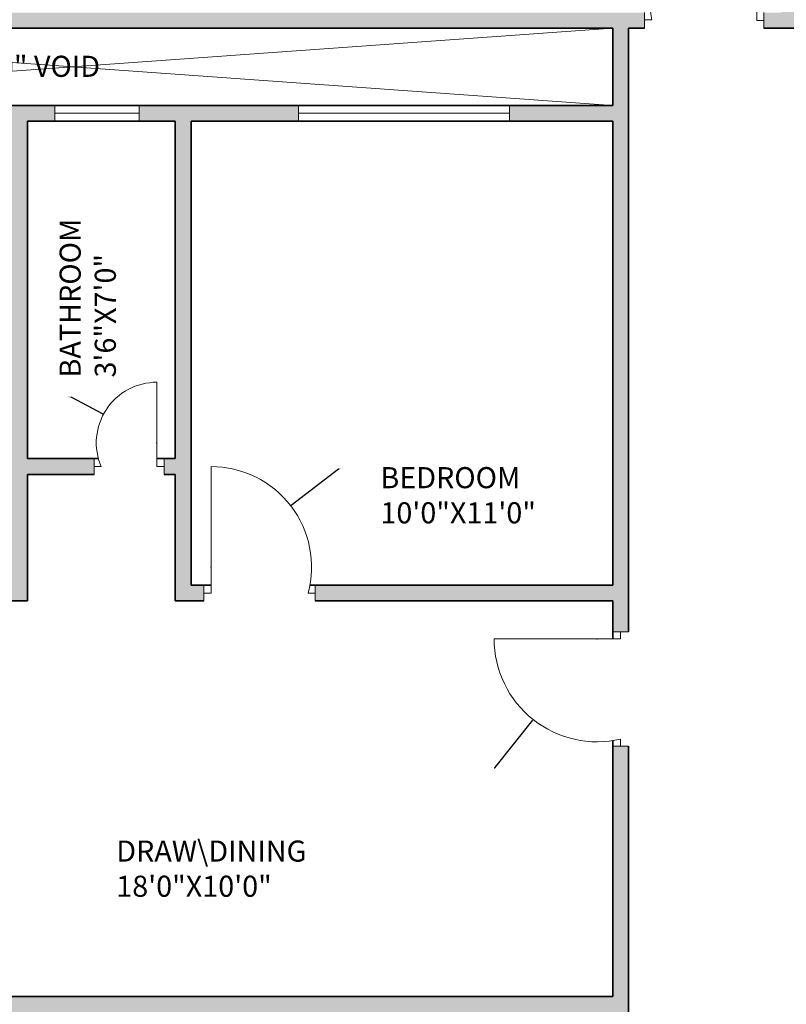
# Model space of a CAD drawing. Units: inches. Extents: x 2314 to 3223, y 1382 to 2735.
# Tile 7 of 14: x 2549 to 2767, y 1864 to 2144. Entities that reach past the tile are written whole.
import ezdxf

# ---------------------------------------------------------------- set-up
doc = ezdxf.new("R2010")
doc.units = ezdxf.units.IN
for name, color, linetype, lineweight in [('A-ANNO-DIMS', 2, 'Continuous', 18), ('A-AREA-IDEN', 7, 'Continuous', 18), ('A-DOOR', 3, 'Continuous', 18), ('A-FLOR-OPEN', 8, 'Continuous', 13), ('A-GLAZ', 4, 'Continuous', 18), ('A-WALL', 7, 'Continuous', 35)]:
    doc.layers.add(name, color=color, linetype=linetype, lineweight=lineweight)
doc.layers.add('A-WALL-PATT', color=251, linetype='Continuous', lineweight=13, true_color=0x636466)
doc.styles.get("Standard").update_dxf_attribs({"font": 'arial.ttf'})
doc.dimstyles.get("Standard").update_dxf_attribs({"dimtxt": 0.18, "dimasz": 0.18, "dimexe": 0.18, "dimexo": 0.0625, "dimgap": 0.09, "dimtad": 0, "dimtih": 1, "dimtoh": 1, "dimdec": 4, "dimzin": 0, "dimdsep": 46, "dimtxsty": 'Standard', "dimcen": 0.09, "dimadec": 0, "dimazin": 0, "dimtfac": 1, "dimtdec": 4, "dimtofl": 0, "dimtmove": 0, "dimatfit": 3, "dimfxl": 1, "dimtolj": 1, "dimtzin": 0, "dimarcsym": 0})

# ---------------------------------------------------------------- blocks, each defined once
blk = doc.blocks.new('WIN-PLAN-24')
for p, q in [((0, 24), (4.5, 24)), ((4.5, 24), (2.25, 24)), ((2.25, 24), (2.25, 0)), ((2.25, 0), (0, 0)), ((0, 0), (4.5, 0))]:
    blk.add_line(p, q)
blk = doc.blocks.new('WIN-PLAN-60')
for p, q in [((0, 4.5), (0, 0)), ((60, 2.25), (60, 4.5)), ((60, 4.5), (60, 0)), ((0, 0), (0, 2.25)), ((0, 2.25), (60, 2.25))]:
    blk.add_line(p, q)
blk = doc.blocks.new('*D70')
at = {"layer": 'A-ANNO-DIMS', "color": 0, "lineweight": -2, "transparency": 16777216}
for p, q in [((2713.37, 1968.13), (2713.55, 1968.13)), ((2713.46, 1968.04), (2713.46, 1968.22)), ((2684.32, 1931.38), (2695.13, 1945.02)), ((2684.14, 1931.38), (2684.32, 1931.38))]:
    blk.add_line(p, q, dxfattribs=at)
at = {"layer": 'A-ANNO-DIMS', "color": 0, "transparency": 16777216}
blk.add_solid([(2695.11, 1945.04), (2695.16, 1945), (2695.24, 1945.16)], dxfattribs=at)
at = {"layer": 'Defpoints', "color": 0, "transparency": 16777216}
for p in [(2713.46, 1968.13), (2695.24, 1945.16)]:
    blk.add_point(p, dxfattribs=at)
at = {"layer": 'A-ANNO-DIMS', "color": 0, "transparency": 16777216, "insert": (2683.59, 1931.38), "char_height": 0.18, "attachment_point": 5}
blk.add_mtext('\\A1;R29.315', dxfattribs=at)
blk = doc.blocks.new('*D72')
at = {"layer": 'A-ANNO-DIMS', "color": 0, "lineweight": -2, "transparency": 16777216}
for p, q in [((2639.91, 2016.41), (2626.43, 2006.06)), ((2640.09, 2016.41), (2639.91, 2016.41)), ((2603.5, 1988.51), (2603.68, 1988.51)), ((2603.59, 1988.42), (2603.59, 1988.6))]:
    blk.add_line(p, q, dxfattribs=at)
at = {"layer": 'A-ANNO-DIMS', "color": 0, "transparency": 16777216}
blk.add_solid([(2626.41, 2006.08), (2626.45, 2006.03), (2626.29, 2005.95)], dxfattribs=at)
at = {"layer": 'Defpoints', "color": 0, "transparency": 16777216}
for p in [(2626.29, 2005.95), (2603.59, 1988.51)]:
    blk.add_point(p, dxfattribs=at)
at = {"layer": 'A-ANNO-DIMS', "color": 0, "transparency": 16777216, "insert": (2640.57, 2016.41), "char_height": 0.18, "attachment_point": 5}
blk.add_mtext('\\A1;R28.62', dxfattribs=at)
blk = doc.blocks.new('*D92')
at = {"layer": 'A-ANNO-DIMS', "color": 0, "lineweight": -2, "transparency": 16777216}
for p, q in [((2563.67, 2036.89), (2563.85, 2036.89)), ((2563.85, 2036.89), (2572.83, 2032.09)), ((2588.12, 2023.87), (2588.3, 2023.87)), ((2588.21, 2023.78), (2588.21, 2023.96))]:
    blk.add_line(p, q, dxfattribs=at)
at = {"layer": 'A-ANNO-DIMS', "color": 0, "transparency": 16777216}
blk.add_solid([(2572.84, 2032.12), (2572.81, 2032.07), (2572.98, 2032.01)], dxfattribs=at)
at = {"layer": 'Defpoints', "color": 0, "transparency": 16777216}
for p in [(2572.98, 2032.01), (2588.21, 2023.87)]:
    blk.add_point(p, dxfattribs=at)
at = {"layer": 'A-ANNO-DIMS', "color": 0, "transparency": 16777216, "insert": (2563.12, 2036.89), "char_height": 0.18, "attachment_point": 5}
blk.add_mtext('\\A1;R17.268', dxfattribs=at)

msp = doc.modelspace()

# ---------------------------------------------------------------- hatches: boundary and pattern name
at = {"layer": 'A-WALL-PATT'}
h = msp.add_hatch(color=256, dxfattribs=at)
h.dxf.hatch_style = 1
h.paths.add_polyline_path([(2443.3302, 2379.5332), (2443.3302, 2381.7832), (2410.3927, 2381.7832), (2410.3927, 2336.7008), (2414.8927, 2336.7008), (2414.8927, 2377.2832), (2443.3302, 2377.2832)])
h.paths.add_polyline_path([(2561.3645, 2379.5332), (2561.3645, 2381.7832), (2503.3302, 2381.7832), (2503.3302, 2377.2832), (2546.8927, 2377.2832), (2546.8927, 2245.2832), (2541.8787, 2245.2832), (2541.8787, 2240.7832), (2551.3927, 2240.7832), (2551.3927, 2377.2832), (2561.3645, 2377.2832)])
h.paths.add_polyline_path([(2656.0607, 2381.7832), (2597.3645, 2381.7832), (2597.3645, 2377.2832), (2617.3927, 2377.2832), (2617.3927, 2257.2832), (2584.2532, 2257.2832), (2584.2532, 2252.7832), (2625.8528, 2252.7832), (2625.8528, 2255.0332), (2625.8528, 2257.2832), (2621.8927, 2257.2832), (2621.8927, 2377.2832), (2656.0607, 2377.2832), (2656.0607, 2379.5332)])
h.paths.add_polyline_path([(2807.3418, 2381.7832), (2716.0607, 2381.7832), (2716.0607, 2377.2832), (2765.8927, 2377.2832), (2765.8927, 2257.2832), (2661.6935, 2257.2832), (2661.6935, 2252.7832), (2765.8927, 2252.7832), (2765.8927, 2146.2832), (2760.9259, 2146.2832), (2760.9259, 2141.8832), (2775.7119, 2141.8832), (2775.7119, 2146.2832), (2770.3927, 2146.2832), (2770.3927, 2252.7832), (2877.684, 2252.7832), (2877.684, 2255.0332), (2877.684, 2257.2832), (2770.3927, 2257.2832), (2770.3927, 2377.2832), (2807.3418, 2377.2832), (2807.3418, 2379.5332)])
h.paths.add_polyline_path([(2937.2118, 2381.7832), (2867.3418, 2381.7832), (2867.3418, 2377.2832), (2914.3927, 2377.2832), (2914.3927, 2257.2832), (2908.4124, 2257.2832), (2908.4124, 2252.7832), (2960.6432, 2252.7832), (2960.6432, 2255.0332), (2960.6432, 2257.2832), (2918.8927, 2257.2832), (2918.8927, 2377.2832), (2937.2118, 2377.2832)])
h.paths.add_polyline_path([(3022.1601, 2381.7832), (2973.2118, 2381.7832), (2973.2118, 2379.5332), (2973.2118, 2377.2832), (2984.8927, 2377.2832), (2984.8927, 2257.2832), (2980.0601, 2257.2832), (2980.0601, 2252.7832), (2984.8927, 2252.7832), (2984.8927, 2240.7832), (2995.668, 2240.7832), (2995.668, 2243.0332), (2995.668, 2245.2832), (2989.3927, 2245.2832), (2989.3927, 2377.2832), (3022.1601, 2377.2832), (3022.1601, 2379.5332)])
h.paths.add_polyline_path([(3125.8927, 2381.7832), (3082.1601, 2381.7832), (3082.1601, 2377.2832), (3121.3927, 2377.2832), (3121.3927, 2334.7388), (3125.8927, 2334.7388)])
h.paths.add_polyline_path([(3125.8927, 2274.7388), (3121.3927, 2274.7388), (3121.3927, 2245.2832), (3066.4832, 2245.2832), (3066.4832, 2240.7832), (3121.3927, 2240.7832), (3121.3927, 2232.1868), (3125.8927, 2232.1868)])
h.paths.add_polyline_path([(3125.8927, 2208.1868), (3121.3927, 2208.1868), (3121.3927, 2198.7832), (3037.3927, 2198.7832), (3037.3927, 2240.7832), (3041.2694, 2240.7832), (3041.2694, 2243.0332), (3041.2694, 2245.2832), (3026.8205, 2245.2832), (3026.8205, 2240.7832), (3032.8927, 2240.7832), (3032.8927, 2190.4022), (3037.3927, 2190.4022), (3037.3927, 2194.2832), (3121.3927, 2194.2832), (3121.3927, 2182.1835), (3125.8927, 2182.1835)])
h.paths.add_polyline_path([(3125.8927, 2158.1835), (3121.3927, 2158.1835), (3121.3927, 2146.2832), (3037.3927, 2146.2832), (3037.3927, 2169.3726), (3035.1427, 2169.3726), (3032.8927, 2169.3726), (3032.8927, 2146.2832), (2812.7301, 2146.2832), (2812.7301, 2144.0832), (2812.7301, 2141.8832), (2818.3927, 2141.8832), (2818.3927, 1970.1316), (2822.8927, 1970.1316), (2822.8927, 1978.8832), (2903.9846, 1978.8832), (2903.9846, 1981.1332), (2903.9846, 1983.3832), (2822.8927, 1983.3832), (2822.8927, 2115.3832), (2851.7162, 2115.3832), (2851.7162, 2117.6332), (2851.7162, 2119.8832), (2822.8927, 2119.8832), (2822.8927, 2141.8832), (3125.8927, 2141.8832)])
h.paths.add_polyline_path([(3125.8927, 2119.8832), (3081.193, 2119.8832), (3081.193, 2115.3832), (3121.3927, 2115.3832), (3121.3927, 2071.8188), (3125.8927, 2071.8188)], flags=17)
h.paths.add_polyline_path([(2989.3927, 2115.3832), (3021.193, 2115.3832), (3021.193, 2117.6332), (3021.193, 2119.8832), (2979.123, 2119.8832), (2979.123, 2115.3832), (2984.8927, 2115.3832), (2984.8927, 2019.3832), (2981.9225, 2019.3832), (2981.9225, 2014.8832), (2984.8927, 2014.8832), (2984.8927, 1983.3832), (2984.8927, 1978.8832), (2989.3927, 1978.8832), (2989.3927, 1983.3832)], flags=17)
h.paths.add_polyline_path([(2947.3927, 2115.3832), (2955.123, 2115.3832), (2955.123, 2117.6332), (2955.123, 2119.8832), (2911.7162, 2119.8832), (2911.7162, 2115.3832), (2942.8927, 2115.3832), (2942.8927, 1983.3832), (2936.7017, 1983.3832), (2936.7017, 1978.8832), (2947.3927, 1978.8832), (2947.3927, 1983.3832), (2947.3927, 2014.8832), (2960.7167, 2014.8832), (2960.7167, 2017.1332), (2960.7167, 2019.3832), (2947.3927, 2019.3832)], flags=17)
h.paths.add_polyline_path([(3037.3927, 1978.8832), (3041.8276, 1978.8832), (3041.8276, 1981.1332), (3041.8276, 1983.3832), (3025.477, 1983.3832), (3025.477, 1978.8832), (3032.8927, 1978.8832), (3032.8927, 1927.1259), (3035.1427, 1927.1259), (3037.3927, 1927.1259)])
h.paths.add_polyline_path([(3125.8927, 2011.8188), (3123.6427, 2011.8188), (3121.3927, 2011.8188), (3121.3927, 1983.3832), (3065, 1983.3832), (3065, 1978.8832), (3121.3927, 1978.8832), (3121.3927, 1970.5932), (3125.8927, 1970.5932)], flags=17)
h.paths.add_polyline_path([(2994.2341, 1983.3832), (2989.3927, 1983.3832), (2989.3927, 1978.8832), (2994.2341, 1978.8832), (2994.2341, 1981.1332)], flags=16)
h.paths.add_polyline_path([(3125.8927, 1946.5932), (3121.3927, 1946.5932), (3121.3927, 1936.8832), (3037.3927, 1936.8832), (3037.3927, 1932.3832), (3121.3927, 1932.3832), (3121.3927, 1919.825), (3125.8927, 1919.825)])
h.paths.add_polyline_path([(3125.8927, 1883.825), (3121.3927, 1883.825), (3121.3927, 1866.3832), (3037.3927, 1866.3832), (3037.3927, 1899.0954), (3035.1427, 1899.0954), (3032.8927, 1899.0954), (3032.8927, 1866.3832), (2822.8927, 1866.3832), (2822.8927, 1938.7212), (2820.6427, 1938.7212), (2818.3927, 1938.7212), (2818.3927, 1786.9239), (2822.8927, 1786.9239), (2822.8927, 1861.8832), (3032.8927, 1861.8832), (3032.8927, 1825.1023), (3037.3927, 1825.1023), (3037.3927, 1861.8832), (3121.3927, 1861.8832), (3121.3927, 1844.6765), (3125.8927, 1844.6765)])
h.paths.add_polyline_path([(3125.8927, 1808.6765), (3121.3927, 1808.6765), (3121.3927, 1795.8832), (3037.3927, 1795.8832), (3037.3927, 1799.4755), (3032.8927, 1799.4755), (3032.8927, 1749.3832), (3026.5034, 1749.3832), (3026.5034, 1744.8832), (3032.8927, 1744.8832), (3034.9255, 1744.8832), (3043.1326, 1744.8832), (3043.1326, 1747.1332), (3043.1326, 1749.3832), (3037.3927, 1749.3832), (3037.3927, 1791.3832), (3121.3927, 1791.3832), (3121.3927, 1783.3103), (3125.8927, 1783.3103)])
h.paths.add_polyline_path([(3125.8927, 1759.3103), (3121.3927, 1759.3103), (3121.3927, 1749.3832), (3065.1845, 1749.3832), (3065.1845, 1744.8832), (3121.3927, 1744.8832), (3121.3927, 1709.3573), (3125.8927, 1709.3573)])
h.paths.add_polyline_path([(3125.8927, 1649.3573), (3121.3927, 1649.3573), (3121.3927, 1612.8832), (3095.116, 1612.8832), (3095.116, 1608.3832), (3125.8927, 1608.3832)])
h.paths.add_polyline_path([(3035.116, 1612.8832), (2993.8927, 1612.8832), (2993.8927, 1744.8832), (2998.7409, 1744.8832), (2998.7409, 1749.3832), (2989.3927, 1749.3832), (2989.3927, 1744.8832), (2989.3927, 1701.3832), (2972.8226, 1701.3832), (2972.8226, 1696.8832), (2989.3927, 1696.8832), (2989.3927, 1612.8832), (2978.2225, 1612.8832), (2978.2225, 1608.3832), (3035.116, 1608.3832), (3035.116, 1610.6332)])
h.paths.add_polyline_path([(2947.3927, 1696.8832), (2950.7566, 1696.8832), (2950.7566, 1699.1332), (2950.7566, 1701.3832), (2947.3927, 1701.3832), (2947.3927, 1744.8832), (2947.3927, 1749.3832), (2937.649, 1749.3832), (2937.649, 1744.8832), (2942.8927, 1744.8832), (2942.8927, 1612.8832), (2907.783, 1612.8832), (2907.783, 1608.3832), (2954.2225, 1608.3832), (2954.2225, 1610.6332), (2954.2225, 1612.8832), (2947.3927, 1612.8832)])
h.paths.add_polyline_path([(2822.8927, 1744.8832), (2905.3491, 1744.8832), (2905.3491, 1747.1332), (2905.3491, 1749.3832), (2822.8927, 1749.3832), (2822.8927, 1756.9185), (2818.3927, 1756.9185), (2818.3927, 1612.8832), (2818.3927, 1569.1205), (2722.3927, 1569.1205), (2722.3927, 1612.8832), (2722.3927, 1756.9185), (2717.8927, 1756.9185), (2717.8927, 1750.0143), (2633.6297, 1750.0143), (2633.6437, 1745.2665), (2717.8927, 1745.5143), (2717.8927, 1612.8832), (2689.8467, 1612.8832), (2689.8467, 1608.3832), (2717.8927, 1608.3832), (2717.8927, 1564.6205), (2722.3927, 1564.6205), (2822.8927, 1564.6205), (2822.8927, 1569.1205), (2822.8927, 1608.3832), (2847.783, 1608.3832), (2847.783, 1610.6332), (2847.783, 1612.8832), (2822.8927, 1612.8832)])
h.paths.add_polyline_path([(2629.8467, 1612.8832), (2597.8927, 1612.8832), (2597.8927, 1744.8832), (2597.8927, 1745.1613), (2601.5887, 1745.1721), (2601.5816, 1747.5932), (2601.5745, 1750.0143), (2593.3927, 1750.0143), (2593.3927, 1744.8832), (2593.3927, 1713.3832), (2589.7588, 1713.3832), (2589.7588, 1708.8832), (2593.3927, 1708.8832), (2593.3927, 1612.8832), (2582.3793, 1612.8832), (2582.3793, 1608.3832), (2629.8467, 1608.3832), (2629.8467, 1610.6332)])
h.paths.add_polyline_path([(2551.3927, 1708.8832), (2567.6776, 1708.8832), (2567.6776, 1711.1332), (2567.6776, 1713.3832), (2551.3927, 1713.3832), (2551.3927, 1744.8832), (2551.3927, 1750.0143), (2543.5657, 1750.0143), (2543.5657, 1747.5079), (2543.5657, 1745.0014), (2546.8927, 1745.0112), (2546.8927, 1744.8832), (2546.8927, 1612.8832), (2502.9339, 1612.8832), (2502.9339, 1608.3832), (2558.3793, 1608.3832), (2558.3793, 1610.6332), (2558.3793, 1612.8832), (2551.3927, 1612.8832)])
h.paths.add_polyline_path([(2414.8927, 1656.2547), (2410.3927, 1656.2547), (2410.3927, 1608.3832), (2442.9339, 1608.3832), (2442.9339, 1610.6332), (2442.9339, 1612.8832), (2414.8927, 1612.8832)])
h.paths.add_polyline_path([(2414.8927, 1744.8832), (2468.8906, 1744.8832), (2468.8906, 1747.1332), (2468.8906, 1749.3832), (2414.8927, 1749.3832), (2414.8927, 1757.7622), (2410.3927, 1757.7622), (2410.3927, 1716.2547), (2414.8927, 1716.2547)])
h.paths.add_polyline_path([(2414.8927, 1791.3832), (2498.8927, 1791.3832), (2498.8927, 1749.3832), (2492.9799, 1749.3832), (2492.9799, 1744.8832), (2498.8927, 1744.8832), (2503.3927, 1744.8832), (2508.0135, 1744.8968), (2508.0059, 1747.4556), (2507.9984, 1750.0143), (2503.3927, 1750.0143), (2503.3927, 1802.6362), (2501.1427, 1802.6362), (2498.8927, 1802.6362), (2498.8927, 1795.8832), (2414.8927, 1795.8832), (2414.8927, 1808.0943), (2410.3927, 1808.0943), (2410.3927, 1781.7622), (2414.8927, 1781.7622)])
h.paths.add_polyline_path([(2722.3927, 1937.589), (2720.1427, 1937.589), (2717.8927, 1937.589), (2717.8927, 1866.3832), (2503.3927, 1866.3832), (2503.3927, 1896.3484), (2498.8927, 1896.3484), (2498.8927, 1866.3832), (2414.8927, 1866.3832), (2414.8927, 1882.1496), (2410.3927, 1882.1496), (2410.3927, 1844.0943), (2414.8927, 1844.0943), (2414.8927, 1861.8832), (2498.8927, 1861.8832), (2498.8927, 1831.4783), (2501.1427, 1831.4783), (2503.3927, 1831.4783), (2503.3927, 1861.8832), (2717.8927, 1861.8832), (2717.8927, 1786.9239), (2722.3927, 1786.9239)])
h.paths.add_polyline_path([(2414.8927, 1932.3832), (2498.8927, 1932.3832), (2498.8927, 1924.7883), (2503.3927, 1924.7883), (2503.3927, 1978.8832), (2505.8599, 1978.8832), (2505.8599, 1981.1332), (2505.8599, 1983.3832), (2493.3697, 1983.3832), (2493.3697, 1978.8832), (2498.8927, 1978.8832), (2498.8927, 1936.8832), (2414.8927, 1936.8832), (2414.8927, 1943.2834), (2410.3927, 1943.2834), (2410.3927, 1918.1496), (2414.8927, 1918.1496)])
h.paths.add_polyline_path([(2414.8927, 2020.3133), (2412.6427, 2020.3133), (2410.3927, 2020.3133), (2410.3927, 1967.2834), (2414.8927, 1967.2834), (2414.8927, 1978.8832), (2468.8513, 1978.8832), (2468.8513, 1981.1332), (2468.8513, 1983.3832), (2414.8927, 1983.3832)])
h.paths.add_polyline_path([(2414.8927, 2115.3832), (2453.004, 2115.3832), (2453.004, 2117.6332), (2453.004, 2119.8832), (2410.3927, 2119.8832), (2410.3927, 2080.3133), (2414.8927, 2080.3133)], flags=17)
h.paths.add_polyline_path([(2559.0969, 2117.6332), (2559.0969, 2119.8832), (2513.004, 2119.8832), (2513.004, 2115.3832), (2546.8927, 2115.3832), (2546.8927, 1983.3832), (2542.7531, 1983.3832), (2542.7531, 1978.8832), (2551.3927, 1978.8832), (2551.3927, 2014.8832), (2570.3098, 2014.8832), (2570.3098, 2017.1332), (2570.3098, 2019.3832), (2551.3927, 2019.3832), (2551.3927, 2115.3832), (2559.0969, 2115.3832)], flags=17)
h.paths.add_polyline_path([(2628.5073, 2117.6332), (2628.5073, 2119.8832), (2583.0969, 2119.8832), (2583.0969, 2115.3832), (2593.3927, 2115.3832), (2593.3927, 2019.3832), (2590.2108, 2019.3832), (2590.2108, 2014.8832), (2593.3927, 2014.8832), (2593.3927, 1978.8832), (2601.5907, 1978.8832), (2601.5907, 1981.1332), (2601.5907, 1983.3832), (2597.8927, 1983.3832), (2597.8927, 2115.3832), (2628.5073, 2115.3832)], flags=17)
h.paths.add_polyline_path([(2722.3927, 2141.8832), (2726.9871, 2141.8832), (2726.9871, 2144.2705), (2726.9871, 2146.2832), (2503.3927, 2146.2832), (2503.3927, 2168.2161), (2501.1427, 2168.2161), (2498.8927, 2168.2161), (2498.8927, 2146.2832), (2414.8927, 2146.2832), (2414.8927, 2156.5041), (2410.3927, 2156.5041), (2410.3927, 2141.8832), (2717.8927, 2141.8832), (2717.8927, 2119.8832), (2688.5073, 2119.8832), (2688.5073, 2115.3832), (2717.8927, 2115.3832), (2717.8927, 1983.3832), (2633.2454, 1983.3832), (2633.2454, 1978.8832), (2717.8927, 1978.8832), (2717.8927, 1970.1316), (2720.1427, 1970.1316), (2722.3927, 1970.1316)])
h.paths.add_polyline_path([(2557.3704, 1462.9278), (2940.0934, 1462.9278), (2940.0934, 1512.3848), (2557.3704, 1512.3848)], flags=9)
h.paths.add_polyline_path([(2846.2527, 1703.1384), (2892.8612, 1703.1384), (2892.8612, 1725.5272), (2846.2527, 1725.5272)], flags=25)
h.paths.add_polyline_path([(2885.6102, 1812.1147), (2946.1505, 1812.1147), (2946.1505, 1834.5035), (2885.6102, 1834.5035)], flags=25)
h.paths.add_polyline_path([(2885.6102, 1884.183), (2946.1505, 1884.183), (2946.1505, 1906.5718), (2885.6102, 1906.5718)], flags=25)
h.paths.add_polyline_path([(3066.365, 1705.5431), (3112.9735, 1705.5431), (3112.9735, 1727.9319), (3066.365, 1727.9319)], flags=9)
h.paths.add_polyline_path([(3061.8255, 1887.7513), (3101.6154, 1887.7513), (3101.6154, 1910.1401), (3061.8255, 1910.1401)], flags=25)
h.paths.add_polyline_path([(3063.3679, 1816.2121), (3103.1578, 1816.2121), (3103.1578, 1838.6009), (3063.3679, 1838.6009)], flags=25)
h.paths.add_polyline_path([(3053.3743, 1768.416), (3107.1329, 1768.416), (3107.1329, 1790.8048), (3053.3743, 1790.8048)], flags=25)
h.paths.add_polyline_path([(3061.6068, 1943.822), (3115.3653, 1943.822), (3115.3653, 1966.2109), (3061.6068, 1966.2109)], flags=9)
h.paths.add_polyline_path([(2745.0978, 1763.6604), (2797.9354, 1763.6604), (2797.9354, 1776.0247), (2745.0978, 1776.0247)], flags=9)
h.paths.add_polyline_path([(2574.2135, 1819.2586), (2634.7538, 1819.2586), (2634.7538, 1841.6474), (2574.2135, 1841.6474)], flags=25)
h.paths.add_polyline_path([(2574.2135, 1891.3269), (2634.7538, 1891.3269), (2634.7538, 1913.7157), (2574.2135, 1913.7157)], flags=25)
h.paths.add_polyline_path([(2638.4466, 1702.43), (2685.0551, 1702.43), (2685.0551, 1724.8188), (2638.4466, 1724.8188)], flags=25)
h.paths.add_polyline_path([(2435.9715, 1697.1215), (2482.5799, 1697.1215), (2482.5799, 1719.5103), (2435.9715, 1719.5103)], flags=9)
h.paths.add_polyline_path([(2431.2046, 1893.7833), (2470.9945, 1893.7833), (2470.9945, 1916.1721), (2431.2046, 1916.1721)], flags=25)
h.paths.add_polyline_path([(2439.8144, 1817.2116), (2479.6043, 1817.2116), (2479.6043, 1839.6004), (2439.8144, 1839.6004)], flags=25)
h.paths.add_polyline_path([(2441.2607, 1753.0942), (2495.0192, 1753.0942), (2495.0192, 1775.483), (2441.2607, 1775.483)], flags=25)
h.paths.add_polyline_path([(2421.216, 1945.3109), (2474.9746, 1945.3109), (2474.9746, 1967.6997), (2421.216, 1967.6997)], flags=25)
h.paths.add_polyline_path([(2585.4464, 1627.5703), (2585.4464, 1679), (2563.0576, 1679), (2563.0576, 1627.5703)], flags=9)
h.paths.add_polyline_path([(2978.3497, 1618.7039), (2978.3497, 1670.1337), (2955.9609, 1670.1337), (2955.9609, 1618.7039)], flags=9)
h.paths.add_polyline_path([(2975.9502, 2041.7828), (2975.9502, 2093.2125), (2953.5614, 2093.2125), (2953.5614, 2041.7828)], flags=25)
h.paths.add_polyline_path([(2835.6537, 1989.2068), (2882.2621, 1989.2068), (2882.2621, 2011.5956), (2835.6537, 2011.5956)], flags=25)
h.paths.add_polyline_path([(2649.3769, 1997.5659), (2695.9853, 1997.5659), (2695.9853, 2019.9547), (2649.3769, 2019.9547)], flags=25)
h.paths.add_polyline_path([(2579.9087, 2040.3429), (2579.9087, 2091.7726), (2557.5198, 2091.7726), (2557.5198, 2040.3429)], flags=25)
h.paths.add_polyline_path([(2783.2404, 1883.1956), (2783.2404, 2067.1369), (2764.694, 2067.1369), (2764.694, 1883.1956)], flags=9)
h.paths.add_polyline_path([(3055.8435, 1993.5571), (3102.4519, 1993.5571), (3102.4519, 2015.9459), (3055.8435, 2015.9459)], flags=25)
h.paths.add_polyline_path([(2423.6009, 1984.6082), (2470.2094, 1984.6082), (2470.2094, 2006.997), (2423.6009, 2006.997)], flags=25)
h.paths.add_polyline_path([(2973.4115, 2123.1668), (3013.1319, 2123.1668), (3013.1319, 2135.531), (2973.4115, 2135.531)], flags=25)
h.paths.add_polyline_path([(2534.3846, 2124.6231), (2574.105, 2124.6231), (2574.105, 2136.9874), (2534.3846, 2136.9874)], flags=25)
h.paths.add_polyline_path([(2829.1368, 2188.1931), (2889.411, 2188.1931), (2889.411, 2210.5819), (2829.1368, 2210.5819)], flags=9)
h.paths.add_polyline_path([(2633.2547, 2185.0437), (2693.5289, 2185.0437), (2693.5289, 2207.4325), (2633.2547, 2207.4325)], flags=9)
h.paths.add_polyline_path([(2445.1812, 2167.0395), (2496.611, 2167.0395), (2496.611, 2189.4284), (2445.1812, 2189.4284)], flags=9)
h.paths.add_polyline_path([(2429.1678, 2194.5482), (2480.5975, 2194.5482), (2480.5975, 2216.937), (2429.1678, 2216.937)], flags=9)
h.paths.add_polyline_path([(3060.1138, 2158.1056), (3111.5436, 2158.1056), (3111.5436, 2180.4944), (3060.1138, 2180.4944)], flags=9)
h.paths.add_polyline_path([(3055.6824, 2201.2631), (3107.1122, 2201.2631), (3107.1122, 2223.652), (3055.6824, 2223.652)], flags=25)
h.paths.add_polyline_path([(3044.3482, 2257.7345), (3090.9567, 2257.7345), (3090.9567, 2280.1233), (3044.3482, 2280.1233)], flags=9)
h.paths.add_polyline_path([(2942.5437, 2306.9625), (2982.3336, 2306.9625), (2982.3336, 2329.3513), (2942.5437, 2329.3513)], flags=9)
h.paths.add_polyline_path([(2799.5865, 2259.1663), (2846.195, 2259.1663), (2846.195, 2281.5551), (2799.5865, 2281.5551)], flags=25)
h.paths.add_polyline_path([(2670.4998, 2261.1493), (2717.1082, 2261.1493), (2717.1082, 2283.5381), (2670.4998, 2283.5381)], flags=25)
h.paths.add_polyline_path([(2553.0333, 2302.7735), (2592.8232, 2302.7735), (2592.8232, 2325.1624), (2553.0333, 2325.1624)], flags=9)
h.paths.add_polyline_path([(2432.0288, 2268.6489), (2478.6372, 2268.6489), (2478.6372, 2291.0377), (2432.0288, 2291.0377)], flags=9)
h = msp.add_hatch(color=256, dxfattribs=at)
h.dxf.hatch_style = 1
h.paths.add_polyline_path([(2503.3927, 2240.7832), (2507.7952, 2240.7832), (2507.7952, 2245.2832), (2496.4262, 2245.2832), (2496.4262, 2243.0332), (2496.4262, 2240.7832), (2498.8927, 2240.7832), (2498.8927, 2198.7832), (2414.8927, 2198.7832), (2414.8927, 2206.5718), (2410.3927, 2206.5718), (2410.3927, 2180.5041), (2412.6427, 2180.5041), (2414.8927, 2180.5041), (2414.8927, 2194.2832), (2498.8927, 2194.2832), (2498.8927, 2191.0069), (2503.3927, 2191.0069)])
h.paths.add_polyline_path([(2414.8927, 2276.7008), (2410.3927, 2276.7008), (2410.3927, 2230.5718), (2414.8927, 2230.5718), (2414.8927, 2240.7832), (2474.2564, 2240.7832), (2474.2564, 2243.0332), (2474.2564, 2245.2832), (2414.8927, 2245.2832)])
h.paths.add_polyline_path([(2557.3704, 1462.9278), (2940.0934, 1462.9278), (2940.0934, 1512.3848), (2557.3704, 1512.3848)], flags=9)
h.paths.add_polyline_path([(2846.2527, 1703.1384), (2892.8612, 1703.1384), (2892.8612, 1725.5272), (2846.2527, 1725.5272)], flags=9)
h.paths.add_polyline_path([(2885.6102, 1812.1147), (2946.1505, 1812.1147), (2946.1505, 1834.5035), (2885.6102, 1834.5035)], flags=9)
h.paths.add_polyline_path([(2885.6102, 1884.183), (2946.1505, 1884.183), (2946.1505, 1906.5718), (2885.6102, 1906.5718)], flags=9)
h.paths.add_polyline_path([(3066.365, 1705.5431), (3112.9735, 1705.5431), (3112.9735, 1727.9319), (3066.365, 1727.9319)], flags=9)
h.paths.add_polyline_path([(3061.8255, 1887.7513), (3101.6154, 1887.7513), (3101.6154, 1910.1401), (3061.8255, 1910.1401)], flags=9)
h.paths.add_polyline_path([(3063.3679, 1816.2121), (3103.1578, 1816.2121), (3103.1578, 1838.6009), (3063.3679, 1838.6009)], flags=9)
h.paths.add_polyline_path([(3053.3743, 1768.416), (3107.1329, 1768.416), (3107.1329, 1790.8048), (3053.3743, 1790.8048)], flags=9)
h.paths.add_polyline_path([(3061.6068, 1943.822), (3115.3653, 1943.822), (3115.3653, 1966.2109), (3061.6068, 1966.2109)], flags=9)
h.paths.add_polyline_path([(2745.0978, 1763.6604), (2797.9354, 1763.6604), (2797.9354, 1776.0247), (2745.0978, 1776.0247)], flags=9)
h.paths.add_polyline_path([(2574.2135, 1819.2586), (2634.7538, 1819.2586), (2634.7538, 1841.6474), (2574.2135, 1841.6474)], flags=9)
h.paths.add_polyline_path([(2574.2135, 1891.3269), (2634.7538, 1891.3269), (2634.7538, 1913.7157), (2574.2135, 1913.7157)], flags=9)
h.paths.add_polyline_path([(2638.4466, 1702.43), (2685.0551, 1702.43), (2685.0551, 1724.8188), (2638.4466, 1724.8188)], flags=9)
h.paths.add_polyline_path([(2435.9715, 1697.1215), (2482.5799, 1697.1215), (2482.5799, 1719.5103), (2435.9715, 1719.5103)], flags=9)
h.paths.add_polyline_path([(2431.2046, 1893.7833), (2470.9945, 1893.7833), (2470.9945, 1916.1721), (2431.2046, 1916.1721)], flags=9)
h.paths.add_polyline_path([(2439.8144, 1817.2116), (2479.6043, 1817.2116), (2479.6043, 1839.6004), (2439.8144, 1839.6004)], flags=9)
h.paths.add_polyline_path([(2441.2607, 1753.0942), (2495.0192, 1753.0942), (2495.0192, 1775.483), (2441.2607, 1775.483)], flags=9)
h.paths.add_polyline_path([(2421.216, 1945.3109), (2474.9746, 1945.3109), (2474.9746, 1967.6997), (2421.216, 1967.6997)], flags=9)
h.paths.add_polyline_path([(2585.4464, 1627.5703), (2585.4464, 1679), (2563.0576, 1679), (2563.0576, 1627.5703)], flags=9)
h.paths.add_polyline_path([(2978.3497, 1618.7039), (2978.3497, 1670.1337), (2955.9609, 1670.1337), (2955.9609, 1618.7039)], flags=9)
h.paths.add_polyline_path([(2975.9502, 2041.7828), (2975.9502, 2093.2125), (2953.5614, 2093.2125), (2953.5614, 2041.7828)], flags=9)
h.paths.add_polyline_path([(2835.6537, 1989.2068), (2882.2621, 1989.2068), (2882.2621, 2011.5956), (2835.6537, 2011.5956)], flags=9)
h.paths.add_polyline_path([(2649.3769, 1997.5659), (2695.9853, 1997.5659), (2695.9853, 2019.9547), (2649.3769, 2019.9547)], flags=9)
h.paths.add_polyline_path([(2579.9087, 2040.3429), (2579.9087, 2091.7726), (2557.5198, 2091.7726), (2557.5198, 2040.3429)], flags=9)
h.paths.add_polyline_path([(2783.2404, 1883.1956), (2783.2404, 2067.1369), (2764.694, 2067.1369), (2764.694, 1883.1956)], flags=9)
h.paths.add_polyline_path([(3055.8435, 1993.5571), (3102.4519, 1993.5571), (3102.4519, 2015.9459), (3055.8435, 2015.9459)], flags=9)
h.paths.add_polyline_path([(2423.6009, 1984.6082), (2470.2094, 1984.6082), (2470.2094, 2006.997), (2423.6009, 2006.997)], flags=9)
h.paths.add_polyline_path([(2973.4115, 2123.1668), (3013.1319, 2123.1668), (3013.1319, 2135.531), (2973.4115, 2135.531)], flags=9)
h.paths.add_polyline_path([(2534.3846, 2124.6231), (2574.105, 2124.6231), (2574.105, 2136.9874), (2534.3846, 2136.9874)], flags=9)
h.paths.add_polyline_path([(2829.1368, 2188.1931), (2889.411, 2188.1931), (2889.411, 2210.5819), (2829.1368, 2210.5819)], flags=9)
h.paths.add_polyline_path([(2633.2547, 2185.0437), (2693.5289, 2185.0437), (2693.5289, 2207.4325), (2633.2547, 2207.4325)], flags=9)
h.paths.add_polyline_path([(2445.1812, 2167.0395), (2496.611, 2167.0395), (2496.611, 2189.4284), (2445.1812, 2189.4284)], flags=9)
h.paths.add_polyline_path([(2429.1678, 2208.3022), (2480.5975, 2208.3022), (2480.5975, 2230.691), (2429.1678, 2230.691)], flags=25)
h.paths.add_polyline_path([(3060.1138, 2158.1056), (3111.5436, 2158.1056), (3111.5436, 2180.4944), (3060.1138, 2180.4944)], flags=9)
h.paths.add_polyline_path([(3055.6824, 2201.2631), (3107.1122, 2201.2631), (3107.1122, 2223.652), (3055.6824, 2223.652)], flags=9)
h.paths.add_polyline_path([(3044.3482, 2257.7345), (3090.9567, 2257.7345), (3090.9567, 2280.1233), (3044.3482, 2280.1233)], flags=9)
h.paths.add_polyline_path([(2942.5437, 2306.9625), (2982.3336, 2306.9625), (2982.3336, 2329.3513), (2942.5437, 2329.3513)], flags=9)
h.paths.add_polyline_path([(2799.5865, 2259.1663), (2846.195, 2259.1663), (2846.195, 2281.5551), (2799.5865, 2281.5551)], flags=9)
h.paths.add_polyline_path([(2670.4998, 2261.1493), (2717.1082, 2261.1493), (2717.1082, 2283.5381), (2670.4998, 2283.5381)], flags=9)
h.paths.add_polyline_path([(2553.0333, 2302.7735), (2592.8232, 2302.7735), (2592.8232, 2325.1624), (2553.0333, 2325.1624)], flags=9)
h.paths.add_polyline_path([(2432.0288, 2268.6489), (2478.6372, 2268.6489), (2478.6372, 2291.0377), (2432.0288, 2291.0377)], flags=9)

# ---------------------------------------------------------------- linework, layer by layer
at = {"layer": 'A-DOOR'}
for p, q in [((2758.9259, 2144.0832), (2758.9259, 2180.0832)), ((2726.9871, 2146.2832), (2726.9871, 2144.2705)), ((2760.9259, 2146.2832), (2760.9259, 2141.8832)), ((2726.9871, 2144.2705), (2726.9871, 2141.8832)), ((2726.9871, 2141.8832), (2726.9871, 2144.2705)), ((2726.9871, 2144.2705), (2728.9871, 2144.2705)), ((2760.9259, 2144.0832), (2758.9259, 2144.0832)), ((2760.9259, 2141.8832), (2760.9259, 2144.0832)), ((2588.2108, 2017.1332), (2588.2108, 2041.1332)), ((2570.3098, 2019.3832), (2570.3098, 2014.8832)), ((2570.3098, 2014.8832), (2570.3098, 2017.1332)), ((2570.3098, 2017.1332), (2572.3098, 2017.1332)), ((2590.2108, 2017.1332), (2588.2108, 2017.1332)), ((2590.2108, 2019.3832), (2590.2108, 2014.8832)), ((2590.2108, 2014.8832), (2590.2108, 2017.1332)), ((2603.5907, 1981.1332), (2603.5907, 2017.1332)), ((2601.5907, 1983.3832), (2601.5907, 1978.8832)), ((2633.2454, 1983.3832), (2633.2454, 1983.3832)), ((2633.2454, 1983.3832), (2633.2454, 1978.8832)), ((2601.5907, 1978.8832), (2601.5907, 1981.1332)), ((2601.5907, 1981.1332), (2603.5907, 1981.1332)), ((2633.2454, 1981.1332), (2631.2454, 1981.1332)), ((2633.2454, 1978.8832), (2633.2454, 1981.1332)), ((2722.3927, 1970.1316), (2717.8927, 1970.1316)), ((2717.8927, 1970.1316), (2720.1427, 1970.1316)), ((2720.1427, 1970.1316), (2720.1427, 1968.1316)), ((2720.1427, 1968.1316), (2684.1427, 1968.1316)), ((2720.1427, 1937.589), (2720.1427, 1939.589)), ((2717.8927, 1937.589), (2722.3927, 1937.589)), ((2722.3927, 1937.589), (2720.1427, 1937.589))]:
    msp.add_line(p, q, dxfattribs=at)
for centre, radius, start, end in [((2758.9259, 2149.6627), 30.4205, 90, 190.209835), ((2588.2108, 2023.8657), 17.2675, 90, 202.947898), ((2603.5907, 1988.5113), 28.6219, 345.06179, 90), ((2713.4577, 1968.1316), 29.315, 180, 283.181733)]:
    msp.add_arc(centre, radius, start, end, dxfattribs=at)
at = {"layer": 'A-FLOR-OPEN'}
for p, q in [((2717.8927, 2141.8832), (2410.3927, 2119.8832)), ((2410.3927, 2141.8832), (2717.8927, 2119.8832))]:
    msp.add_line(p, q, dxfattribs=at)
at = {"layer": 'A-WALL'}
for p, q in [((2410.3927, 2141.8832), (2717.8927, 2141.8832)), ((2717.8927, 2141.8832), (2717.8927, 2119.8832)), ((2722.3927, 2141.8832), (2722.3927, 1970.1316)), ((2722.3927, 2141.8832), (2726.9871, 2141.8832)), ((2760.9259, 2141.8832), (2775.7119, 2141.8832)), ((2410.3927, 2119.8832), (2717.8927, 2119.8832)), ((2551.3927, 2115.3832), (2551.3927, 2019.3832)), ((2593.3927, 2115.3832), (2551.3927, 2115.3832)), ((2593.3927, 2115.3832), (2593.3927, 2019.3832)), ((2597.8927, 2115.3832), (2597.8927, 1983.3832)), ((2717.8927, 2115.3832), (2597.8927, 2115.3832)), ((2717.8927, 2115.3832), (2717.8927, 1983.3832)), ((2571.5352, 2019.3832), (2551.3927, 2019.3832)), ((2593.3927, 2019.3832), (2588.2108, 2019.3832)), ((2570.3098, 2014.8832), (2551.3927, 2014.8832)), ((2551.3927, 2014.8832), (2551.3927, 1978.8832)), ((2593.3927, 2014.8832), (2590.2108, 2014.8832)), ((2593.3927, 2014.8832), (2593.3927, 1978.8832)), ((2603.5907, 1983.3832), (2597.8927, 1983.3832)), ((2717.8927, 1983.3832), (2631.7495, 1983.3832)), ((2551.3927, 1978.8832), (2542.7531, 1978.8832)), ((2601.5907, 1978.8832), (2593.3927, 1978.8832)), ((2717.8927, 1978.8832), (2633.2454, 1978.8832)), ((2717.8927, 1978.8832), (2717.8927, 1968.1316)), ((2717.8927, 1939.154), (2717.8927, 1866.3832)), ((2722.3927, 1937.589), (2722.3927, 1786.9239)), ((2717.8927, 1866.3832), (2503.3927, 1866.3832))]:
    msp.add_line(p, q, dxfattribs=at)

# ---------------------------------------------------------------- block references
at = {"layer": 'A-GLAZ', "extrusion": (0, 0, -1), "zscale": -1, "rotation": 90}
msp.add_blockref('WIN-PLAN-24', (-2559.0969, 2115.3832), dxfattribs=at)
at = {"layer": 'A-GLAZ', "rotation": 180}
msp.add_blockref('WIN-PLAN-60', (2688.5073, 2119.8832), dxfattribs=at)

# ---------------------------------------------------------------- texts
at = {"layer": 'A-AREA-IDEN', "char_height": 6, "attachment_point": 1}
for s, width, insert in [('2\'0" VOID', 144.40599, (2536.1302, 2134.0058)), ('BEDROOM\\P10\'0"X11\'0"', 131.289442, (2651.7896, 2016.9731)), ('DRAW\\\\DINING\\P18\'0"X10\'0"', 98.983827, (2576.6262, 1910.7301))]:
    msp.add_mtext_dynamic_manual_height_columns(s, width=width, gutter_width=12.5, heights=[0], dxfattribs=dict(at, insert=insert))
at = {"layer": 'A-AREA-IDEN', "insert": (2560.5014, 2042.4568), "char_height": 6, "attachment_point": 1, "rotation": 90}
msp.add_mtext_dynamic_manual_height_columns('BATHROOM\\P3\'6"X7\'0"', width=102.84301, gutter_width=12.5, heights=[0], dxfattribs=at)

# ---------------------------------------------------------------- dimensions: what is measured, and where the dimension line sits
at = {"layer": 'A-ANNO-DIMS'}
for center, mpoint, override, picture, middle in [((2588.2108, 2023.8657), (2572.9838, 2032.0086), {"dimdec": 3, "dimlfac": 1, "dimrnd": 0, "dimzin": 0, "dimdsep": 46, "dimlunit": 2}, '*D92', (2563.1177, 2036.8944)), ((2603.5907, 1988.5113), (2626.289, 2005.947), {"dimdec": 2, "dimlfac": 1, "dimrnd": 0, "dimzin": 0, "dimdsep": 46, "dimlunit": 2}, '*D72', (2640.5669, 2016.4084)), ((2713.4577, 1968.1316), (2695.2448, 1945.1607), {"dimdec": 3, "dimlfac": 1, "dimrnd": 0, "dimzin": 0, "dimdsep": 46, "dimlunit": 2}, '*D70', (2683.5866, 1931.3782))]:
    dim = msp.add_radius_dim(center=center, mpoint=mpoint, dimstyle='Standard', override=override, dxfattribs=at)
    dim.commit()
    dim.dimension.update_dxf_attribs({"geometry": picture, "text_midpoint": middle, "dimtype": 164})

doc.saveas('drawing.dxf')
